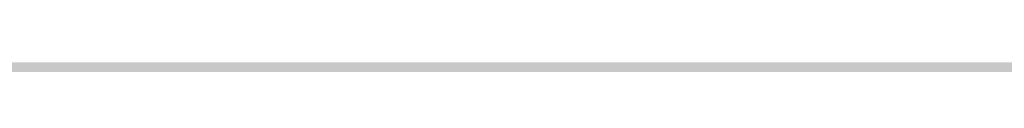
# Model space of a CAD drawing. Units: millimetres. Extents: x 0 to 2267, y 0 to 1823.
# Tile 207 of 256: x 1841.442 to 1842.748, y 1127.414 to 1127.416. Entities that reach past the tile are written whole.
import ezdxf

# ---------------------------------------------------------------- set-up
doc = ezdxf.new("R2010")
doc.units = ezdxf.units.MM
doc.header["$MEASUREMENT"] = 0
doc.layers.add('M-DIMS', color=2, linetype='Continuous', lineweight=25)
doc.layers.add('M-HATC', color=252, linetype='Continuous', lineweight=18)
doc.styles.get("Standard").update_dxf_attribs({"font": 'arial.ttf'})
doc.dimstyles.get("Standard").update_dxf_attribs({"dimtxt": 7, "dimasz": 4, "dimexe": 0.18, "dimexo": 0.0625, "dimgap": 0.09, "dimtad": 0, "dimdec": 0, "dimzin": 0, "dimdsep": 46, "dimtxsty": 'Standard', "dimcen": 0.09, "dimadec": 0, "dimazin": 0, "dimtfac": 1, "dimtdec": 0, "dimtofl": 0, "dimtmove": 0, "dimatfit": 3, "dimfxl": 1, "dimtolj": 1, "dimtzin": 0, "dimarcsym": 0})

# ---------------------------------------------------------------- blocks, each defined once
blk = doc.blocks.new('*D1')
at = {"layer": 'Defpoints', "color": 0, "transparency": 16777216}
for p in [(1593.4289, 1127.4171), (1843.4289, 1127.4171), (1843.4289, 955.6278)]:
    blk.add_point(p, dxfattribs=at)
at = {"layer": 'M-DIMS', "color": 0, "lineweight": -2, "transparency": 16777216}
for p, q in [((1593.4289, 1127.3546), (1593.4289, 955.4478)), ((1843.4289, 1127.3546), (1843.4289, 955.4478)), ((1597.4289, 955.6278), (1710.5582, 955.6278)), ((1839.4289, 955.6278), (1726.2996, 955.6278))]:
    blk.add_line(p, q, dxfattribs=at)
at = {"layer": 'M-DIMS', "color": 0, "transparency": 16777216}
for points in [[(1597.4289, 956.2944), (1597.4289, 954.9611), (1593.4289, 955.6278)], [(1839.4289, 956.2944), (1839.4289, 954.9611), (1843.4289, 955.6278)]]:
    blk.add_solid(points, dxfattribs=at)
at = {"layer": 'M-DIMS', "color": 0, "transparency": 16777216, "insert": (1718.4289, 955.6278), "char_height": 7, "attachment_point": 5}
blk.add_mtext('\\A1;250', dxfattribs=at)

msp = doc.modelspace()

# ---------------------------------------------------------------- hatches: boundary and pattern name
at = {"layer": 'M-HATC'}
h = msp.add_hatch(color=256, dxfattribs=at)
h.dxf.hatch_style = 1
h.paths.add_polyline_path([(2055.771, 1603.062), (1381.0868, 1603.062), (1381.0868, 1598.062), (2055.771, 1598.062)])
h.paths.add_polyline_path([(2055.771, 1598.062), (1381.0868, 1598.062), (1381.0868, 1593.062), (2055.771, 1593.062)])
h.paths.add_polyline_path([(2051.3074, 1536.7609), (1385.5504, 1536.7609), (1385.5504, 1526.7609), (1387.5504, 1526.7609), (1388.5366, 1525.0528), (1385.3319, 1521.2335), (1385.3319, 1521.2226), (2050.2542, 1522.7491), (2048.3212, 1525.0528), (2049.3074, 1526.7609), (2051.3074, 1526.7609)])
edge = h.paths.add_edge_path()
edge.add_arc((1847.5345, 1379.1492), 135, 222.603061, 222.890851, ccw=False)
edge.add_line((1748.1663, 1287.7656), (1683.0921, 1287.7656))
edge.add_arc((1583.7239, 1379.1492), 135, 317.109149, 317.396939, ccw=False)
edge.add_arc((1678.9686, 1290.6707), 5, 222.8909, 317.1091, ccw=False)
edge.add_arc((1774.2133, 1379.1492), 135, 222.603061, 222.890851, ccw=False)
edge.add_line((1674.8451, 1287.7656), (1609.7709, 1287.7656))
edge.add_arc((1510.4027, 1379.1492), 135, 317.109149, 317.396939, ccw=False)
edge.add_arc((1605.6474, 1290.6707), 5, 222.8909, 317.1091, ccw=False)
edge.add_arc((1700.8921, 1379.1492), 135, 222.603061, 222.890851, ccw=False)
edge.add_line((1601.5239, 1287.7656), (1536.4497, 1287.7656))
edge.add_arc((1437.0815, 1379.1492), 135, 317.109149, 317.396939, ccw=False)
edge.add_arc((1532.3262, 1290.6707), 5, 222.8909, 317.1091, ccw=False)
edge.add_arc((1627.5709, 1379.1492), 135, 222.603061, 222.890851, ccw=False)
edge.add_line((1528.2027, 1287.7656), (1505.9289, 1287.7656))
edge.add_spline(control_points=[(1505.9289, 1287.7656), (1504.2622, 1287.7656), (1504.2622, 1282.7656), (1505.9289, 1282.7656)], knot_values=[0, 0, 0, 0, 5, 5, 5, 5], degree=3, periodic=0)
edge.add_line((1505.9289, 1282.7656), (1930.9289, 1282.7656))
edge.add_spline(control_points=[(1930.9289, 1282.7656), (1932.5956, 1282.7656), (1932.5956, 1287.7656), (1930.9289, 1287.7656)], knot_values=[0, 0, 0, 0, 5, 5, 5, 5], degree=3, periodic=0)
edge.add_line((1930.9289, 1287.7656), (1903.0557, 1287.7656))
edge.add_arc((1803.6875, 1379.1492), 135, 317.109149, 317.396939, ccw=False)
edge.add_arc((1898.9322, 1290.6707), 5, 222.8909, 317.1091, ccw=False)
edge.add_arc((1994.1769, 1379.1492), 135, 222.603061, 222.890851, ccw=False)
edge.add_line((1894.8087, 1287.7656), (1829.7345, 1287.7656))
edge.add_arc((1730.3663, 1379.1492), 135, 317.109149, 317.396939, ccw=False)
edge.add_arc((1825.611, 1290.6707), 5, 222.8909, 317.1091, ccw=False)
edge.add_arc((1920.8557, 1379.1492), 135, 222.603061, 222.890851, ccw=False)
edge.add_line((1821.4875, 1287.7656), (1756.4133, 1287.7656))
edge.add_arc((1657.0451, 1379.1492), 135, 317.109149, 317.396939, ccw=False)
edge.add_arc((1752.2898, 1290.6707), 5, 222.8909, 317.1091, ccw=False)
edge = h.paths.add_edge_path()
edge.add_spline(control_points=[(1843.4289, 1227.2475), (1845.0956, 1227.2475), (1845.0956, 1232.2475), (1843.4289, 1232.2475)], knot_values=[0, 0, 0, 0, 5, 5, 5, 5], degree=3, periodic=0)
edge.add_line((1843.4289, 1232.2475), (1593.4289, 1232.2475))
edge.add_spline(control_points=[(1593.4289, 1232.2475), (1591.7622, 1232.2475), (1591.7622, 1227.2475), (1593.4289, 1227.2475)], knot_values=[0, 0, 0, 0, 5, 5, 5, 5], degree=3, periodic=0)
edge.add_line((1593.4289, 1227.2475), (1843.4289, 1227.2475))
h.paths.add_polyline_path([(1905.9289, 1127.4171), (1530.9289, 1127.4171, 0.414214), (1520.9289, 1117.4171), (1530.9289, 1117.4171), (1915.9289, 1117.4171, 0.414214)])
edge = h.paths.add_edge_path()
edge.add_arc((1397.0858, 1498.4078), 12.7299, 90.78215, 190.87871, ccw=False)
edge.add_line((1396.912, 1511.1365), (1428.0097, 1511.3488))
edge.add_line((1428.0097, 1511.3488), (1433.0097, 1511.3488))
edge.add_line((1433.0097, 1511.3488), (1434.439, 1511.3488))
edge.add_arc((1419.474, 1498.0804), 20, 41.561, 74.08211)
edge.add_line((1424.9592, 1517.3135), (1399.9351, 1517.2561))
edge.add_spline(control_points=[(1399.9307, 1517.2561), (1399.884, 1517.2131), (1399.8328, 1517.1689), (1399.7774, 1517.1236)], knot_values=[11.567499, 11.567499, 11.567499, 11.567499, 11.814249, 11.814249, 11.814249, 11.814249], degree=3, periodic=0)
edge.add_spline(control_points=[(1399.6328, 1517.0099), (1399.5831, 1516.9721), (1399.5307, 1516.9338), (1399.4759, 1516.8947)], knot_values=[11.167718, 11.167718, 11.167718, 11.167718, 11.365188, 11.365188, 11.365188, 11.365188], degree=3, periodic=0)
edge.add_spline(control_points=[(1399.3398, 1516.8001), (1399.1514, 1516.6719), (1398.9384, 1516.5377), (1398.704, 1516.3994)], knot_values=[10.376405, 10.376405, 10.376405, 10.376405, 11.00994, 11.00994, 11.00994, 11.00994], degree=3, periodic=0)
edge.add_spline(control_points=[(1398.6572, 1516.3719), (1398.5789, 1516.326), (1398.4983, 1516.2797), (1398.4155, 1516.2331)], knot_values=[10.125175, 10.125175, 10.125175, 10.125175, 10.334406, 10.334406, 10.334406, 10.334406], degree=3, periodic=0)
edge.add_spline(control_points=[(1398.2642, 1516.1487), (1398.196, 1516.1111), (1398.1263, 1516.0732), (1398.0555, 1516.0351)], knot_values=[9.832246, 9.832246, 9.832246, 9.832246, 9.999658, 9.999658, 9.999658, 9.999658], degree=3, periodic=0)
edge.add_spline(control_points=[(1397.9987, 1516.0048), (1397.7312, 1515.8621), (1397.446, 1515.7171), (1397.1466, 1515.5714)], knot_values=[9.161808, 9.161808, 9.161808, 9.161808, 9.787769, 9.787769, 9.787769, 9.787769], degree=3, periodic=0)
edge.add_spline(control_points=[(1397.1466, 1515.5714), (1396.8418, 1515.423), (1396.5222, 1515.274), (1396.1914, 1515.1262)], knot_values=[8.524455, 8.524455, 8.524455, 8.524455, 9.161808, 9.161808, 9.161808, 9.161808], degree=3, periodic=0)
edge.add_spline(control_points=[(1396.0777, 1515.0756), (1395.9854, 1515.0348), (1395.8922, 1514.994), (1395.7983, 1514.9534)], knot_values=[8.275193, 8.275193, 8.275193, 8.275193, 8.451726, 8.451726, 8.451726, 8.451726], degree=3, periodic=0)
edge.add_spline(control_points=[(1395.6018, 1514.8691), (1395.4997, 1514.8257), (1395.3968, 1514.7824), (1395.2932, 1514.7394)], knot_values=[7.962917, 7.962917, 7.962917, 7.962917, 8.152764, 8.152764, 8.152764, 8.152764], degree=3, periodic=0)
edge.add_spline(control_points=[(1395.2116, 1514.7057), (1394.8278, 1514.5475), (1394.4345, 1514.3929), (1394.0364, 1514.2442)], knot_values=[7.21254, 7.21254, 7.21254, 7.21254, 7.913148, 7.913148, 7.913148, 7.913148], degree=3, periodic=0)
edge.add_spline(control_points=[(1394.0364, 1514.2442), (1393.7076, 1514.1214), (1393.3754, 1514.0027), (1393.0427, 1513.8895)], knot_values=[6.633733, 6.633733, 6.633733, 6.633733, 7.21254, 7.21254, 7.21254, 7.21254], degree=3, periodic=0)
edge.add_spline(control_points=[(1392.8214, 1513.815), (1392.7198, 1513.7812), (1392.6181, 1513.7479), (1392.5166, 1513.7152)], knot_values=[6.328796, 6.328796, 6.328796, 6.328796, 6.505493, 6.505493, 6.505493, 6.505493], degree=3, periodic=0)
edge.add_spline(control_points=[(1392.5166, 1513.7152), (1392.3187, 1513.6515), (1392.1212, 1513.59), (1391.9244, 1513.531)], knot_values=[5.984605, 5.984605, 5.984605, 5.984605, 6.328796, 6.328796, 6.328796, 6.328796], degree=3, periodic=0)
edge.add_spline(control_points=[(1391.7915, 1513.4915), (1391.3122, 1513.3501), (1390.8384, 1513.2239), (1390.3784, 1513.1171)], knot_values=[5.066697, 5.066697, 5.066697, 5.066697, 5.907055, 5.907055, 5.907055, 5.907055], degree=3, periodic=0)
edge.add_spline(control_points=[(1390.3784, 1513.1171), (1390.1797, 1513.071), (1389.9836, 1513.0284), (1389.7907, 1512.9899)], knot_values=[4.70367, 4.70367, 4.70367, 4.70367, 5.066695, 5.066695, 5.066695, 5.066695], degree=3, periodic=0)
edge.add_spline(control_points=[(1389.422, 1512.9204), (1389.2459, 1512.8892), (1389.0729, 1512.8617), (1388.9036, 1512.8381)], knot_values=[4.130571, 4.130571, 4.130571, 4.130571, 4.469816, 4.469816, 4.469816, 4.469816], degree=3, periodic=0)
edge.add_spline(control_points=[(1388.9036, 1512.8381), (1388.591, 1512.7946), (1388.2911, 1512.7644), (1388.0071, 1512.7494)], knot_values=[3.504031, 3.504031, 3.504031, 3.504031, 4.130571, 4.130571, 4.130571, 4.130571], degree=3, periodic=0)
edge.add_spline(control_points=[(1387.9356, 1512.7459), (1387.8538, 1512.7423), (1387.7733, 1512.74), (1387.6944, 1512.739)], knot_values=[3.268866, 3.268866, 3.268866, 3.268866, 3.451164, 3.451164, 3.451164, 3.451164], degree=3, periodic=0)
edge.add_spline(control_points=[(1387.3351, 1512.7443), (1387.2076, 1512.7499), (1387.0847, 1512.7597), (1386.967, 1512.7739)], knot_values=[2.670686, 2.670686, 2.670686, 2.670686, 2.984, 2.984, 2.984, 2.984], degree=3, periodic=0)
edge.add_spline(control_points=[(1386.8327, 1512.7922), (1386.8209, 1512.7941), (1386.8092, 1512.7959), (1386.7975, 1512.7979)], knot_values=[2.516981, 2.516981, 2.516981, 2.516981, 2.549528, 2.549528, 2.549528, 2.549528], degree=3, periodic=0)
edge.add_spline(control_points=[(1386.4526, 1512.8735), (1386.4257, 1512.881), (1386.3993, 1512.889), (1386.3733, 1512.8972)], knot_values=[2.095869, 2.095869, 2.095869, 2.095869, 2.17941, 2.17941, 2.17941, 2.17941], degree=3, periodic=0)
edge.add_spline(control_points=[(1386.0691, 1513.0189), (1386.0634, 1513.0217), (1386.0577, 1513.0246), (1386.052, 1513.0275)], knot_values=[1.72453, 1.72453, 1.72453, 1.72453, 1.745933, 1.745933, 1.745933, 1.745933], degree=3, periodic=0)
edge.add_arc((1399.474, 1498.0804), 20, 131.82432, 180)
edge.add_arc((1630.3336, 1505.5484), 250.9708, 181.705176, 236.427975)
edge.add_arc((1605.3399, 1483.3044), 218.7822, 238.660829, 243.34961)
edge.add_arc((1647.0911, 1510.3592), 262.8986, 183.129836, 237.853442, ccw=False)
h.paths.add_polyline_path([(1406.5369, 1391.9644, 0.149382), (1491.5506, 1296.4418, -0.129517)], flags=17)
edge = h.paths.add_edge_path()
edge.add_arc((2037.3838, 1498.0804), 20, 0, 48.26587)
edge.add_spline(control_points=[(2050.6973, 1513.0052), (2050.6512, 1512.9847), (2050.6034, 1512.9655), (2050.5539, 1512.9477)], knot_values=[1.835652, 1.835652, 1.835652, 1.835652, 2.000781, 2.000781, 2.000781, 2.000781], degree=3, periodic=0)
edge.add_spline(control_points=[(2050.4616, 1512.9166), (2050.479, 1512.9221), (2050.4963, 1512.9277), (2050.5133, 1512.9335)], knot_values=[2.045477, 2.045477, 2.045477, 2.045477, 2.101389, 2.101389, 2.101389, 2.101389], degree=3, periodic=0)
edge.add_spline(control_points=[(2050.129, 1512.8342), (2050.1984, 1512.8473), (2050.2657, 1512.8623), (2050.3308, 1512.8792)], knot_values=[2.237629, 2.237629, 2.237629, 2.237629, 2.435841, 2.435841, 2.435841, 2.435841], degree=3, periodic=0)
edge.add_spline(control_points=[(2050.0946, 1512.8278), (2050.1061, 1512.8299), (2050.1176, 1512.832), (2050.129, 1512.8342)], knot_values=[2.435841, 2.435841, 2.435841, 2.435841, 2.468321, 2.468321, 2.468321, 2.468321], degree=3, periodic=0)
edge.add_spline(control_points=[(2049.7843, 1512.7851), (2049.8552, 1512.7922), (2049.9243, 1512.8008), (2049.9917, 1512.8109)], knot_values=[2.563852, 2.563852, 2.563852, 2.563852, 2.748541, 2.748541, 2.748541, 2.748541], degree=3, periodic=0)
edge.add_spline(control_points=[(2049.4052, 1512.7617), (2049.5364, 1512.7653), (2049.6629, 1512.773), (2049.7843, 1512.7851)], knot_values=[2.748541, 2.748541, 2.748541, 2.748541, 3.064882, 3.064882, 3.064882, 3.064882], degree=3, periodic=0)
edge.add_spline(control_points=[(2049.1698, 1512.7597), (2049.2336, 1512.7591), (2049.2965, 1512.7594), (2049.3584, 1512.7606)], knot_values=[3.102309, 3.102309, 3.102309, 3.102309, 3.2503, 3.2503, 3.2503, 3.2503], degree=3, periodic=0)
edge.add_spline(control_points=[(2048.8573, 1512.7691), (2048.9638, 1512.7638), (2049.068, 1512.7606), (2049.1698, 1512.7597)], knot_values=[3.2503, 3.2503, 3.2503, 3.2503, 3.486069, 3.486069, 3.486069, 3.486069], degree=3, periodic=0)
edge.add_spline(control_points=[(2048.6924, 1512.7789), (2048.3729, 1512.8009), (2048.0345, 1512.8411), (2047.6817, 1512.897)], knot_values=[3.606429, 3.606429, 3.606429, 3.606429, 4.2989, 4.2989, 4.2989, 4.2989], degree=3, periodic=0)
edge.add_spline(control_points=[(2047.6817, 1512.897), (2047.5458, 1512.9185), (2047.4077, 1512.9424), (2047.2678, 1512.9685)], knot_values=[4.2989, 4.2989, 4.2989, 4.2989, 4.565769, 4.565769, 4.565769, 4.565769], degree=3, periodic=0)
edge.add_spline(control_points=[(2047.2678, 1512.9685), (2047.1449, 1512.9914), (2047.0207, 1513.016), (2046.8951, 1513.0422)], knot_values=[4.565769, 4.565769, 4.565769, 4.565769, 4.799971, 4.799971, 4.799971, 4.799971], degree=3, periodic=0)
edge.add_spline(control_points=[(2046.8951, 1513.0422), (2046.5286, 1513.1188), (2046.1513, 1513.209), (2045.7676, 1513.3107)], knot_values=[4.799971, 4.799971, 4.799971, 4.799971, 5.483718, 5.483718, 5.483718, 5.483718], degree=3, periodic=0)
edge.add_spline(control_points=[(2045.7676, 1513.3107), (2045.3724, 1513.4154), (2044.9704, 1513.5322), (2044.5662, 1513.6588)], knot_values=[5.483718, 5.483718, 5.483718, 5.483718, 6.187866, 6.187866, 6.187866, 6.187866], degree=3, periodic=0)
edge.add_spline(control_points=[(2044.5662, 1513.6588), (2044.4149, 1513.7061), (2044.2633, 1513.7549), (2044.1116, 1513.8048)], knot_values=[6.187866, 6.187866, 6.187866, 6.187866, 6.451551, 6.451551, 6.451551, 6.451551], degree=3, periodic=0)
edge.add_spline(control_points=[(2044.1116, 1513.8048), (2043.9967, 1513.8427), (2043.8817, 1513.8813), (2043.7668, 1513.9205)], knot_values=[6.451551, 6.451551, 6.451551, 6.451551, 6.651434, 6.651434, 6.651434, 6.651434], degree=3, periodic=0)
edge.add_spline(control_points=[(2043.7668, 1513.9205), (2043.3716, 1514.0554), (2042.9774, 1514.1979), (2042.5886, 1514.3458)], knot_values=[6.651434, 6.651434, 6.651434, 6.651434, 7.338879, 7.338879, 7.338879, 7.338879], degree=3, periodic=0)
edge.add_spline(control_points=[(2042.5886, 1514.3458), (2042.1643, 1514.5071), (2041.7465, 1514.6749), (2041.3409, 1514.846)], knot_values=[7.338879, 7.338879, 7.338879, 7.338879, 8.089209, 8.089209, 8.089209, 8.089209], degree=3, periodic=0)
edge.add_spline(control_points=[(2041.3409, 1514.846), (2041.1028, 1514.9465), (2040.869, 1515.0481), (2040.6405, 1515.1502)], knot_values=[8.089209, 8.089209, 8.089209, 8.089209, 8.529587, 8.529587, 8.529587, 8.529587], degree=3, periodic=0)
edge.add_spline(control_points=[(2040.51, 1515.2089), (2040.0824, 1515.4022), (2039.6747, 1515.5971), (2039.295, 1515.7894)], knot_values=[8.613818, 8.613818, 8.613818, 8.613818, 9.44571, 9.44571, 9.44571, 9.44571], degree=3, periodic=0)
edge.add_spline(control_points=[(2039.295, 1515.7894), (2039.0618, 1515.9075), (2038.8391, 1516.0246), (2038.6288, 1516.1398)], knot_values=[9.44571, 9.44571, 9.44571, 9.44571, 9.956404, 9.956404, 9.956404, 9.956404], degree=3, periodic=0)
edge.add_spline(control_points=[(2038.6288, 1516.1398), (2038.5187, 1516.2001), (2038.4121, 1516.2598), (2038.309, 1516.3189)], knot_values=[9.956404, 9.956404, 9.956404, 9.956404, 10.223542, 10.223542, 10.223542, 10.223542], degree=3, periodic=0)
edge.add_spline(control_points=[(2038.309, 1516.3189), (2038.2138, 1516.3735), (2038.1216, 1516.4276), (2038.0328, 1516.481)], knot_values=[10.223542, 10.223542, 10.223542, 10.223542, 10.47051, 10.47051, 10.47051, 10.47051], degree=3, periodic=0)
edge.add_spline(control_points=[(2038.0328, 1516.481), (2037.7855, 1516.6296), (2037.5639, 1516.773), (2037.3722, 1516.909)], knot_values=[10.47051, 10.47051, 10.47051, 10.47051, 11.15767, 11.15767, 11.15767, 11.15767], degree=3, periodic=0)
edge.add_spline(control_points=[(2037.3722, 1516.909), (2037.2789, 1516.9752), (2037.1927, 1517.0396), (2037.1142, 1517.102)], knot_values=[11.15767, 11.15767, 11.15767, 11.15767, 11.49227, 11.49227, 11.49227, 11.49227], degree=3, periodic=0)
edge.add_spline(control_points=[(2036.8564, 1517.3259), (2036.9148, 1517.2692), (2036.9814, 1517.2103), (2037.0557, 1517.1492)], knot_values=[11.577341, 11.577341, 11.577341, 11.577341, 11.91035, 11.91035, 11.91035, 11.91035], degree=3, periodic=0)
edge.add_spline(control_points=[(2036.8074, 1517.3748), (2036.823, 1517.3587), (2036.8393, 1517.3424), (2036.8564, 1517.3259)], knot_values=[11.91035, 11.91035, 11.91035, 11.91035, 12.007402, 12.007402, 12.007402, 12.007402], degree=3, periodic=0)
edge.add_spline(control_points=[(2036.7017, 1517.494), (2036.7104, 1517.483), (2036.7196, 1517.4719), (2036.7291, 1517.4606)], knot_values=[12.184155, 12.184155, 12.184155, 12.184155, 12.255409, 12.255409, 12.255409, 12.255409], degree=3, periodic=0)
edge.add_spline(control_points=[(2036.6159, 1517.6205), (2036.62, 1517.613), (2036.6243, 1517.6055), (2036.6289, 1517.5979)], knot_values=[12.487913, 12.487913, 12.487913, 12.487913, 12.541035, 12.541035, 12.541035, 12.541035], degree=3, periodic=0)
edge.add_spline(control_points=[(2036.5635, 1517.786), (2036.5637, 1517.7794), (2036.5642, 1517.7726), (2036.565, 1517.7658)], knot_values=[12.911761, 12.911761, 12.911761, 12.911761, 12.968286, 12.968286, 12.968286, 12.968286], degree=3, periodic=0)
edge.add_spline(control_points=[(2036.6166, 1517.9304), (2036.6125, 1517.9259), (2036.6086, 1517.9212), (2036.6049, 1517.9165)], knot_values=[13.382527, 13.382527, 13.382527, 13.382527, 13.433791, 13.433791, 13.433791, 13.433791], degree=3, periodic=0)
edge.add_spline(control_points=[(2036.749, 1518.017), (2036.7361, 1518.0116), (2036.7239, 1518.006), (2036.7124, 1518.0002)], knot_values=[13.726299, 13.726299, 13.726299, 13.726299, 13.809928, 13.809928, 13.809928, 13.809928], degree=3, periodic=0)
edge.add_spline(control_points=[(2036.8604, 1518.0528), (2036.8386, 1518.0474), (2036.8181, 1518.0416), (2036.7988, 1518.0353)], knot_values=[13.910887, 13.910887, 13.910887, 13.910887, 14.02153, 14.02153, 14.02153, 14.02153], degree=3, periodic=0)
edge.add_line((2036.9639, 1518.0804), (2032.3838, 1518.0804))
edge.add_line((2032.3838, 1518.0804), (2027.3838, 1518.0804))
edge.add_line((2027.3838, 1518.0804), (2022.3838, 1518.0804))
edge.add_line((2022.3838, 1518.0804), (2017.3838, 1518.0804))
edge.add_arc((2017.3838, 1498.0804), 20, 90, 138.439)
edge.add_line((2002.4188, 1511.3488), (2003.8481, 1511.3488))
edge.add_line((2003.8481, 1511.3488), (2008.8481, 1511.3488))
edge.add_line((2008.8481, 1511.3488), (2039.772, 1511.1377))
edge.add_arc((2039.772, 1498.4078), 12.7299, -10.87871, 90, ccw=False)
edge.add_arc((1789.7668, 1510.3592), 262.8986, 302.146558, 356.870164, ccw=False)
edge.add_arc((1831.5179, 1483.3044), 218.7822, 296.65039, 301.339171)
edge.add_arc((1806.5242, 1505.5484), 250.9708, 303.572025, 358.294824)
h.paths.add_polyline_path([(2030.321, 1391.9644, -0.129517), (1945.3072, 1296.4418, 0.149382)], flags=17)
edge = h.paths.add_edge_path()
edge.add_spline(control_points=[(2037.2464, 1518.0821), (2037.2898, 1518.081), (2037.3355, 1518.0804), (2037.3838, 1518.0804)], knot_values=[0.000012, 0.000012, 0.000012, 0.000012, 0.144754, 0.144754, 0.144754, 0.144754], degree=3, periodic=0)
edge.add_line((2037.3357, 1518.0804), (2037.0096, 1518.0804))
edge.add_spline(control_points=[(2037.0096, 1518.0804), (2036.9822, 1518.0768), (2036.956, 1518.0727), (2036.9312, 1518.0681)], knot_values=[14.13465, 14.13465, 14.13465, 14.13465, 14.247197, 14.247197, 14.247197, 14.247197], degree=3, periodic=0)
edge.add_spline(control_points=[(2036.9312, 1518.0681), (2036.9276, 1518.0674), (2036.9241, 1518.0667), (2036.9205, 1518.0661)], knot_values=[14.118315, 14.118315, 14.118315, 14.118315, 14.13465, 14.13465, 14.13465, 14.13465], degree=3, periodic=0)
edge.add_spline(control_points=[(2036.9205, 1518.0661), (2036.9118, 1518.0644), (2036.9032, 1518.0626), (2036.8948, 1518.0608)], knot_values=[14.078086, 14.078086, 14.078086, 14.078086, 14.118315, 14.118315, 14.118315, 14.118315], degree=3, periodic=0)
edge.add_spline(control_points=[(2036.8948, 1518.0608), (2036.883, 1518.0583), (2036.8716, 1518.0556), (2036.8604, 1518.0528)], knot_values=[14.02153, 14.02153, 14.02153, 14.02153, 14.078086, 14.078086, 14.078086, 14.078086], degree=3, periodic=0)
edge.add_spline(control_points=[(2036.8604, 1518.0528), (2036.8386, 1518.0474), (2036.8181, 1518.0416), (2036.7988, 1518.0353)], knot_values=[13.910887, 13.910887, 13.910887, 13.910887, 14.02153, 14.02153, 14.02153, 14.02153], degree=3, periodic=0)
edge.add_spline(control_points=[(2036.7988, 1518.0353), (2036.7981, 1518.035), (2036.7974, 1518.0348), (2036.7967, 1518.0346)], knot_values=[13.906906, 13.906906, 13.906906, 13.906906, 13.910887, 13.910887, 13.910887, 13.910887], degree=3, periodic=0)
edge.add_spline(control_points=[(2036.7967, 1518.0346), (2036.7882, 1518.0318), (2036.7799, 1518.0289), (2036.7719, 1518.0259)], knot_values=[13.857826, 13.857826, 13.857826, 13.857826, 13.906906, 13.906906, 13.906906, 13.906906], degree=3, periodic=0)
edge.add_spline(control_points=[(2036.7719, 1518.0259), (2036.764, 1518.023), (2036.7564, 1518.02), (2036.749, 1518.017)], knot_values=[13.809928, 13.809928, 13.809928, 13.809928, 13.857826, 13.857826, 13.857826, 13.857826], degree=3, periodic=0)
edge.add_spline(control_points=[(2036.749, 1518.017), (2036.7361, 1518.0116), (2036.7239, 1518.006), (2036.7124, 1518.0002)], knot_values=[13.726299, 13.726299, 13.726299, 13.726299, 13.809928, 13.809928, 13.809928, 13.809928], degree=3, periodic=0)
edge.add_spline(control_points=[(2036.7124, 1518.0002), (2036.7121, 1518), (2036.7118, 1517.9999), (2036.7115, 1517.9997)], knot_values=[13.723993, 13.723993, 13.723993, 13.723993, 13.726299, 13.726299, 13.726299, 13.726299], degree=3, periodic=0)
edge.add_spline(control_points=[(2036.7115, 1517.9997), (2036.7063, 1517.9971), (2036.7013, 1517.9944), (2036.6965, 1517.9917)], knot_values=[13.686536, 13.686536, 13.686536, 13.686536, 13.723993, 13.723993, 13.723993, 13.723993], degree=3, periodic=0)
edge.add_spline(control_points=[(2036.6965, 1517.9917), (2036.6919, 1517.9891), (2036.6874, 1517.9865), (2036.6831, 1517.9839)], knot_values=[13.651251, 13.651251, 13.651251, 13.651251, 13.686536, 13.686536, 13.686536, 13.686536], degree=3, periodic=0)
edge.add_spline(control_points=[(2036.6831, 1517.9839), (2036.6764, 1517.9798), (2036.67, 1517.9757), (2036.6639, 1517.9714)], knot_values=[13.596804, 13.596804, 13.596804, 13.596804, 13.651251, 13.651251, 13.651251, 13.651251], degree=3, periodic=0)
edge.add_spline(control_points=[(2036.6639, 1517.9714), (2036.6636, 1517.9712), (2036.6633, 1517.9709), (2036.6629, 1517.9707)], knot_values=[13.593956, 13.593956, 13.593956, 13.593956, 13.596804, 13.596804, 13.596804, 13.596804], degree=3, periodic=0)
edge.add_spline(control_points=[(2036.6629, 1517.9707), (2036.6603, 1517.9689), (2036.6577, 1517.967), (2036.6552, 1517.9651)], knot_values=[13.570322, 13.570322, 13.570322, 13.570322, 13.593956, 13.593956, 13.593956, 13.593956], degree=3, periodic=0)
edge.add_spline(control_points=[(2036.6552, 1517.9651), (2036.6525, 1517.9631), (2036.6499, 1517.9611), (2036.6474, 1517.9591)], knot_values=[13.545477, 13.545477, 13.545477, 13.545477, 13.570322, 13.570322, 13.570322, 13.570322], degree=3, periodic=0)
edge.add_spline(control_points=[(2036.6474, 1517.9591), (2036.6472, 1517.9589), (2036.6471, 1517.9588), (2036.6469, 1517.9587)], knot_values=[13.543931, 13.543931, 13.543931, 13.543931, 13.545477, 13.545477, 13.545477, 13.545477], degree=3, periodic=0)
edge.add_spline(control_points=[(2036.6469, 1517.9587), (2036.6412, 1517.9541), (2036.6358, 1517.9494), (2036.6307, 1517.9447)], knot_values=[13.488237, 13.488237, 13.488237, 13.488237, 13.543931, 13.543931, 13.543931, 13.543931], degree=3, periodic=0)
edge.add_spline(control_points=[(2036.6307, 1517.9447), (2036.6282, 1517.9423), (2036.6257, 1517.9399), (2036.6233, 1517.9374)], knot_values=[13.460307, 13.460307, 13.460307, 13.460307, 13.488237, 13.488237, 13.488237, 13.488237], degree=3, periodic=0)
edge.add_spline(control_points=[(2036.6233, 1517.9374), (2036.6215, 1517.9356), (2036.6198, 1517.9338), (2036.6181, 1517.932)], knot_values=[13.439712, 13.439712, 13.439712, 13.439712, 13.460307, 13.460307, 13.460307, 13.460307], degree=3, periodic=0)
edge.add_spline(control_points=[(2036.6181, 1517.932), (2036.6176, 1517.9315), (2036.6171, 1517.9309), (2036.6166, 1517.9304)], knot_values=[13.433791, 13.433791, 13.433791, 13.433791, 13.439712, 13.439712, 13.439712, 13.439712], degree=3, periodic=0)
edge.add_spline(control_points=[(2036.6166, 1517.9304), (2036.6125, 1517.9259), (2036.6086, 1517.9212), (2036.6049, 1517.9165)], knot_values=[13.382527, 13.382527, 13.382527, 13.382527, 13.433791, 13.433791, 13.433791, 13.433791], degree=3, periodic=0)
edge.add_spline(control_points=[(2036.6049, 1517.9165), (2036.6026, 1517.9135), (2036.6004, 1517.9104), (2036.5982, 1517.9074)], knot_values=[13.350017, 13.350017, 13.350017, 13.350017, 13.382527, 13.382527, 13.382527, 13.382527], degree=3, periodic=0)
edge.add_spline(control_points=[(2036.5982, 1517.9074), (2036.5972, 1517.9059), (2036.5962, 1517.9043), (2036.5952, 1517.9028)], knot_values=[13.333922, 13.333922, 13.333922, 13.333922, 13.350017, 13.350017, 13.350017, 13.350017], degree=3, periodic=0)
edge.add_spline(control_points=[(2036.5952, 1517.9028), (2036.5945, 1517.9018), (2036.5939, 1517.9009), (2036.5933, 1517.8999)], knot_values=[13.323828, 13.323828, 13.323828, 13.323828, 13.333922, 13.333922, 13.333922, 13.333922], degree=3, periodic=0)
edge.add_spline(control_points=[(2036.5933, 1517.8999), (2036.5905, 1517.8955), (2036.5879, 1517.8909), (2036.5855, 1517.8864)], knot_values=[13.277545, 13.277545, 13.277545, 13.277545, 13.323828, 13.323828, 13.323828, 13.323828], degree=3, periodic=0)
edge.add_spline(control_points=[(2036.5855, 1517.8864), (2036.5836, 1517.8827), (2036.5817, 1517.8789), (2036.5801, 1517.8751)], knot_values=[13.240119, 13.240119, 13.240119, 13.240119, 13.277545, 13.277545, 13.277545, 13.277545], degree=3, periodic=0)
edge.add_spline(control_points=[(2036.5801, 1517.8751), (2036.5795, 1517.8739), (2036.579, 1517.8727), (2036.5785, 1517.8715)], knot_values=[13.228211, 13.228211, 13.228211, 13.228211, 13.240119, 13.240119, 13.240119, 13.240119], degree=3, periodic=0)
edge.add_spline(control_points=[(2036.5785, 1517.8715), (2036.578, 1517.8702), (2036.5774, 1517.869), (2036.5769, 1517.8677)], knot_values=[13.215717, 13.215717, 13.215717, 13.215717, 13.228211, 13.228211, 13.228211, 13.228211], degree=3, periodic=0)
edge.add_spline(control_points=[(2036.5769, 1517.8677), (2036.5755, 1517.864), (2036.5741, 1517.8603), (2036.5729, 1517.8565)], knot_values=[13.179847, 13.179847, 13.179847, 13.179847, 13.215717, 13.215717, 13.215717, 13.215717], degree=3, periodic=0)
edge.add_spline(control_points=[(2036.5729, 1517.8565), (2036.5713, 1517.8515), (2036.5699, 1517.8464), (2036.5687, 1517.8413)], knot_values=[13.132017, 13.132017, 13.132017, 13.132017, 13.179847, 13.179847, 13.179847, 13.179847], degree=3, periodic=0)
edge.add_spline(control_points=[(2036.5687, 1517.8413), (2036.5684, 1517.8402), (2036.5682, 1517.8392), (2036.568, 1517.8382)], knot_values=[13.122482, 13.122482, 13.122482, 13.122482, 13.132017, 13.132017, 13.132017, 13.132017], degree=3, periodic=0)
edge.add_spline(control_points=[(2036.568, 1517.8382), (2036.5676, 1517.8363), (2036.5672, 1517.8345), (2036.5669, 1517.8327)], knot_values=[13.105592, 13.105592, 13.105592, 13.105592, 13.122482, 13.122482, 13.122482, 13.122482], degree=3, periodic=0)
edge.add_spline(control_points=[(2036.5669, 1517.8327), (2036.5662, 1517.8292), (2036.5657, 1517.8257), (2036.5652, 1517.8222)], knot_values=[13.074063, 13.074063, 13.074063, 13.074063, 13.105592, 13.105592, 13.105592, 13.105592], degree=3, periodic=0)
edge.add_spline(control_points=[(2036.5652, 1517.8222), (2036.5652, 1517.8222), (2036.5652, 1517.8222), (2036.5652, 1517.8222)], knot_values=[13.074043, 13.074043, 13.074043, 13.074043, 13.074063, 13.074063, 13.074063, 13.074063], degree=3, periodic=0)
edge.add_spline(control_points=[(2036.5652, 1517.8222), (2036.5644, 1517.8164), (2036.5639, 1517.8106), (2036.5636, 1517.8046)], knot_values=[13.021884, 13.021884, 13.021884, 13.021884, 13.074043, 13.074043, 13.074043, 13.074043], degree=3, periodic=0)
edge.add_spline(control_points=[(2036.5636, 1517.8046), (2036.5636, 1517.804), (2036.5636, 1517.8034), (2036.5635, 1517.8028)], knot_values=[13.01674, 13.01674, 13.01674, 13.01674, 13.021884, 13.021884, 13.021884, 13.021884], degree=3, periodic=0)
edge.add_spline(control_points=[(2036.5635, 1517.8028), (2036.5634, 1517.8005), (2036.5634, 1517.7982), (2036.5634, 1517.7958)], knot_values=[12.996438, 12.996438, 12.996438, 12.996438, 13.01674, 13.01674, 13.01674, 13.01674], degree=3, periodic=0)
edge.add_spline(control_points=[(2036.5634, 1517.7958), (2036.5633, 1517.7926), (2036.5634, 1517.7893), (2036.5635, 1517.786)], knot_values=[12.968286, 12.968286, 12.968286, 12.968286, 12.996438, 12.996438, 12.996438, 12.996438], degree=3, periodic=0)
edge.add_spline(control_points=[(2036.5635, 1517.786), (2036.5637, 1517.7794), (2036.5642, 1517.7726), (2036.565, 1517.7658)], knot_values=[12.911761, 12.911761, 12.911761, 12.911761, 12.968286, 12.968286, 12.968286, 12.968286], degree=3, periodic=0)
edge.add_spline(control_points=[(2036.565, 1517.7658), (2036.565, 1517.7657), (2036.565, 1517.7656), (2036.565, 1517.7656)], knot_values=[12.911017, 12.911017, 12.911017, 12.911017, 12.911761, 12.911761, 12.911761, 12.911761], degree=3, periodic=0)
edge.add_spline(control_points=[(2036.565, 1517.7656), (2036.5654, 1517.7625), (2036.5658, 1517.7593), (2036.5663, 1517.7562)], knot_values=[12.88528, 12.88528, 12.88528, 12.88528, 12.911017, 12.911017, 12.911017, 12.911017], degree=3, periodic=0)
edge.add_spline(control_points=[(2036.5663, 1517.7562), (2036.5667, 1517.7534), (2036.5672, 1517.7506), (2036.5677, 1517.7478)], knot_values=[12.862519, 12.862519, 12.862519, 12.862519, 12.88528, 12.88528, 12.88528, 12.88528], degree=3, periodic=0)
edge.add_spline(control_points=[(2036.5677, 1517.7478), (2036.5678, 1517.7474), (2036.5679, 1517.7469), (2036.568, 1517.7465)], knot_values=[12.858885, 12.858885, 12.858885, 12.858885, 12.862519, 12.862519, 12.862519, 12.862519], degree=3, periodic=0)
edge.add_spline(control_points=[(2036.568, 1517.7465), (2036.5692, 1517.7399), (2036.5707, 1517.7332), (2036.5724, 1517.7264)], knot_values=[12.8053, 12.8053, 12.8053, 12.8053, 12.858885, 12.858885, 12.858885, 12.858885], degree=3, periodic=0)
edge.add_spline(control_points=[(2036.5724, 1517.7264), (2036.5734, 1517.7226), (2036.5745, 1517.7187), (2036.5756, 1517.7149)], knot_values=[12.775176, 12.775176, 12.775176, 12.775176, 12.8053, 12.8053, 12.8053, 12.8053], degree=3, periodic=0)
edge.add_spline(control_points=[(2036.5756, 1517.7149), (2036.5763, 1517.7125), (2036.577, 1517.7102), (2036.5778, 1517.7078)], knot_values=[12.756759, 12.756759, 12.756759, 12.756759, 12.775176, 12.775176, 12.775176, 12.775176], degree=3, periodic=0)
edge.add_spline(control_points=[(2036.5778, 1517.7078), (2036.5781, 1517.7067), (2036.5784, 1517.7057), (2036.5787, 1517.7047)], knot_values=[12.748742, 12.748742, 12.748742, 12.748742, 12.756759, 12.756759, 12.756759, 12.756759], degree=3, periodic=0)
edge.add_spline(control_points=[(2036.5787, 1517.7047), (2036.5808, 1517.6983), (2036.5831, 1517.6919), (2036.5856, 1517.6854)], knot_values=[12.69959, 12.69959, 12.69959, 12.69959, 12.748742, 12.748742, 12.748742, 12.748742], degree=3, periodic=0)
edge.add_spline(control_points=[(2036.5856, 1517.6854), (2036.5876, 1517.68), (2036.5898, 1517.6746), (2036.5921, 1517.6692)], knot_values=[12.659038, 12.659038, 12.659038, 12.659038, 12.69959, 12.69959, 12.69959, 12.69959], degree=3, periodic=0)
edge.add_spline(control_points=[(2036.5921, 1517.6692), (2036.594, 1517.6648), (2036.5959, 1517.6605), (2036.5979, 1517.6561)], knot_values=[12.626806, 12.626806, 12.626806, 12.626806, 12.659038, 12.659038, 12.659038, 12.659038], degree=3, periodic=0)
edge.add_spline(control_points=[(2036.5979, 1517.6561), (2036.5984, 1517.6551), (2036.5989, 1517.6541), (2036.5993, 1517.6531)], knot_values=[12.619394, 12.619394, 12.619394, 12.619394, 12.626806, 12.626806, 12.626806, 12.626806], degree=3, periodic=0)
edge.add_spline(control_points=[(2036.5993, 1517.6531), (2036.6043, 1517.6424), (2036.6099, 1517.6315), (2036.6159, 1517.6205)], knot_values=[12.541039, 12.541039, 12.541039, 12.541039, 12.619394, 12.619394, 12.619394, 12.619394], degree=3, periodic=0)
edge.add_spline(control_points=[(2036.6159, 1517.6205), (2036.6159, 1517.6205), (2036.6159, 1517.6205), (2036.6159, 1517.6205)], knot_values=[12.541035, 12.541035, 12.541035, 12.541035, 12.541039, 12.541039, 12.541039, 12.541039], degree=3, periodic=0)
edge.add_spline(control_points=[(2036.6159, 1517.6205), (2036.62, 1517.613), (2036.6243, 1517.6055), (2036.6289, 1517.5979)], knot_values=[12.487913, 12.487913, 12.487913, 12.487913, 12.541035, 12.541035, 12.541035, 12.541035], degree=3, periodic=0)
edge.add_spline(control_points=[(2036.6289, 1517.5979), (2036.6326, 1517.5916), (2036.6365, 1517.5853), (2036.6406, 1517.5789)], knot_values=[12.443982, 12.443982, 12.443982, 12.443982, 12.487913, 12.487913, 12.487913, 12.487913], degree=3, periodic=0)
edge.add_spline(control_points=[(2036.6406, 1517.5789), (2036.6414, 1517.5776), (2036.6423, 1517.5763), (2036.6431, 1517.5749)], knot_values=[12.434996, 12.434996, 12.434996, 12.434996, 12.443982, 12.443982, 12.443982, 12.443982], degree=3, periodic=0)
edge.add_spline(control_points=[(2036.6431, 1517.5749), (2036.6531, 1517.5596), (2036.6639, 1517.5439), (2036.6756, 1517.528)], knot_values=[12.329647, 12.329647, 12.329647, 12.329647, 12.434996, 12.434996, 12.434996, 12.434996], degree=3, periodic=0)
edge.add_spline(control_points=[(2036.6756, 1517.528), (2036.6839, 1517.5168), (2036.6925, 1517.5055), (2036.7017, 1517.494)], knot_values=[12.255409, 12.255409, 12.255409, 12.255409, 12.329647, 12.329647, 12.329647, 12.329647], degree=3, periodic=0)
edge.add_spline(control_points=[(2036.7017, 1517.494), (2036.7104, 1517.483), (2036.7196, 1517.4719), (2036.7291, 1517.4606)], knot_values=[12.184155, 12.184155, 12.184155, 12.184155, 12.255409, 12.255409, 12.255409, 12.255409], degree=3, periodic=0)
edge.add_spline(control_points=[(2036.7291, 1517.4606), (2036.7436, 1517.4435), (2036.759, 1517.4262), (2036.7753, 1517.4085)], knot_values=[12.075961, 12.075961, 12.075961, 12.075961, 12.184155, 12.184155, 12.184155, 12.184155], degree=3, periodic=0)
edge.add_spline(control_points=[(2036.7753, 1517.4085), (2036.7763, 1517.4075), (2036.7773, 1517.4064), (2036.7783, 1517.4054)], knot_values=[12.069502, 12.069502, 12.069502, 12.069502, 12.075961, 12.075961, 12.075961, 12.075961], degree=3, periodic=0)
edge.add_spline(control_points=[(2036.7783, 1517.4054), (2036.7877, 1517.3953), (2036.7974, 1517.385), (2036.8074, 1517.3748)], knot_values=[12.007402, 12.007402, 12.007402, 12.007402, 12.069502, 12.069502, 12.069502, 12.069502], degree=3, periodic=0)
edge.add_spline(control_points=[(2036.8074, 1517.3748), (2036.823, 1517.3587), (2036.8393, 1517.3424), (2036.8564, 1517.3259)], knot_values=[11.91035, 11.91035, 11.91035, 11.91035, 12.007402, 12.007402, 12.007402, 12.007402], degree=3, periodic=0)
edge.add_spline(control_points=[(2036.8564, 1517.3259), (2036.9148, 1517.2692), (2036.9814, 1517.2103), (2037.0557, 1517.1492)], knot_values=[11.577341, 11.577341, 11.577341, 11.577341, 11.91035, 11.91035, 11.91035, 11.91035], degree=3, periodic=0)
edge.add_spline(control_points=[(2037.0557, 1517.1492), (2037.0747, 1517.1336), (2037.0942, 1517.1179), (2037.1142, 1517.102)], knot_values=[11.49227, 11.49227, 11.49227, 11.49227, 11.577341, 11.577341, 11.577341, 11.577341], degree=3, periodic=0)
edge.add_spline(control_points=[(2037.1142, 1517.102), (2037.1927, 1517.0396), (2037.2789, 1516.9752), (2037.3722, 1516.909)], knot_values=[11.15767, 11.15767, 11.15767, 11.15767, 11.49227, 11.49227, 11.49227, 11.49227], degree=3, periodic=0)
edge.add_spline(control_points=[(2037.3722, 1516.909), (2037.5639, 1516.773), (2037.7855, 1516.6296), (2038.0328, 1516.481)], knot_values=[10.47051, 10.47051, 10.47051, 10.47051, 11.15767, 11.15767, 11.15767, 11.15767], degree=3, periodic=0)
edge.add_spline(control_points=[(2038.0328, 1516.481), (2038.1216, 1516.4276), (2038.2138, 1516.3735), (2038.309, 1516.3189)], knot_values=[10.223542, 10.223542, 10.223542, 10.223542, 10.47051, 10.47051, 10.47051, 10.47051], degree=3, periodic=0)
edge.add_spline(control_points=[(2038.309, 1516.3189), (2038.4121, 1516.2598), (2038.5187, 1516.2001), (2038.6288, 1516.1398)], knot_values=[9.956404, 9.956404, 9.956404, 9.956404, 10.223542, 10.223542, 10.223542, 10.223542], degree=3, periodic=0)
edge.add_spline(control_points=[(2038.6288, 1516.1398), (2038.8391, 1516.0246), (2039.0618, 1515.9075), (2039.295, 1515.7894)], knot_values=[9.44571, 9.44571, 9.44571, 9.44571, 9.956404, 9.956404, 9.956404, 9.956404], degree=3, periodic=0)
edge.add_spline(control_points=[(2039.295, 1515.7894), (2039.6747, 1515.5971), (2040.0824, 1515.4022), (2040.51, 1515.2089)], knot_values=[8.613818, 8.613818, 8.613818, 8.613818, 9.44571, 9.44571, 9.44571, 9.44571], degree=3, periodic=0)
edge.add_spline(control_points=[(2040.51, 1515.2089), (2040.5533, 1515.1893), (2040.5968, 1515.1697), (2040.6405, 1515.1502)], knot_values=[8.529587, 8.529587, 8.529587, 8.529587, 8.613818, 8.613818, 8.613818, 8.613818], degree=3, periodic=0)
edge.add_spline(control_points=[(2040.6405, 1515.1502), (2040.869, 1515.0481), (2041.1028, 1514.9465), (2041.3409, 1514.846)], knot_values=[8.089209, 8.089209, 8.089209, 8.089209, 8.529587, 8.529587, 8.529587, 8.529587], degree=3, periodic=0)
edge.add_spline(control_points=[(2041.3409, 1514.846), (2041.7465, 1514.6749), (2042.1643, 1514.5071), (2042.5886, 1514.3458)], knot_values=[7.338879, 7.338879, 7.338879, 7.338879, 8.089209, 8.089209, 8.089209, 8.089209], degree=3, periodic=0)
edge.add_spline(control_points=[(2042.5886, 1514.3458), (2042.9774, 1514.1979), (2043.3716, 1514.0554), (2043.7668, 1513.9205)], knot_values=[6.651434, 6.651434, 6.651434, 6.651434, 7.338879, 7.338879, 7.338879, 7.338879], degree=3, periodic=0)
edge.add_spline(control_points=[(2043.7668, 1513.9205), (2043.8817, 1513.8813), (2043.9967, 1513.8427), (2044.1116, 1513.8048)], knot_values=[6.451551, 6.451551, 6.451551, 6.451551, 6.651434, 6.651434, 6.651434, 6.651434], degree=3, periodic=0)
edge.add_spline(control_points=[(2044.1116, 1513.8048), (2044.2633, 1513.7549), (2044.4149, 1513.7061), (2044.5662, 1513.6588)], knot_values=[6.187866, 6.187866, 6.187866, 6.187866, 6.451551, 6.451551, 6.451551, 6.451551], degree=3, periodic=0)
edge.add_spline(control_points=[(2044.5662, 1513.6588), (2044.9704, 1513.5322), (2045.3724, 1513.4154), (2045.7676, 1513.3107)], knot_values=[5.483718, 5.483718, 5.483718, 5.483718, 6.187866, 6.187866, 6.187866, 6.187866], degree=3, periodic=0)
edge.add_spline(control_points=[(2045.7676, 1513.3107), (2046.1513, 1513.209), (2046.5286, 1513.1188), (2046.8951, 1513.0422)], knot_values=[4.799971, 4.799971, 4.799971, 4.799971, 5.483718, 5.483718, 5.483718, 5.483718], degree=3, periodic=0)
edge.add_spline(control_points=[(2046.8951, 1513.0422), (2047.0207, 1513.016), (2047.1449, 1512.9914), (2047.2678, 1512.9685)], knot_values=[4.565769, 4.565769, 4.565769, 4.565769, 4.799971, 4.799971, 4.799971, 4.799971], degree=3, periodic=0)
edge.add_spline(control_points=[(2047.2678, 1512.9685), (2047.4077, 1512.9424), (2047.5458, 1512.9185), (2047.6817, 1512.897)], knot_values=[4.2989, 4.2989, 4.2989, 4.2989, 4.565769, 4.565769, 4.565769, 4.565769], degree=3, periodic=0)
edge.add_spline(control_points=[(2047.6817, 1512.897), (2048.0345, 1512.8411), (2048.3729, 1512.8009), (2048.6924, 1512.7789)], knot_values=[3.606429, 3.606429, 3.606429, 3.606429, 4.2989, 4.2989, 4.2989, 4.2989], degree=3, periodic=0)
edge.add_spline(control_points=[(2048.6924, 1512.7789), (2048.7479, 1512.7751), (2048.8029, 1512.7718), (2048.8573, 1512.7691)], knot_values=[3.486069, 3.486069, 3.486069, 3.486069, 3.606429, 3.606429, 3.606429, 3.606429], degree=3, periodic=0)
edge.add_spline(control_points=[(2048.8573, 1512.7691), (2048.9638, 1512.7638), (2049.068, 1512.7606), (2049.1698, 1512.7597)], knot_values=[3.2503, 3.2503, 3.2503, 3.2503, 3.486069, 3.486069, 3.486069, 3.486069], degree=3, periodic=0)
edge.add_spline(control_points=[(2049.1698, 1512.7597), (2049.2336, 1512.7591), (2049.2965, 1512.7594), (2049.3584, 1512.7606)], knot_values=[3.102309, 3.102309, 3.102309, 3.102309, 3.2503, 3.2503, 3.2503, 3.2503], degree=3, periodic=0)
edge.add_spline(control_points=[(2049.3584, 1512.7606), (2049.3741, 1512.7609), (2049.3897, 1512.7613), (2049.4052, 1512.7617)], knot_values=[3.064882, 3.064882, 3.064882, 3.064882, 3.102309, 3.102309, 3.102309, 3.102309], degree=3, periodic=0)
edge.add_spline(control_points=[(2049.4052, 1512.7617), (2049.5364, 1512.7653), (2049.6629, 1512.773), (2049.7843, 1512.7851)], knot_values=[2.748541, 2.748541, 2.748541, 2.748541, 3.064882, 3.064882, 3.064882, 3.064882], degree=3, periodic=0)
edge.add_spline(control_points=[(2049.7843, 1512.7851), (2049.8552, 1512.7922), (2049.9243, 1512.8008), (2049.9917, 1512.8109)], knot_values=[2.563852, 2.563852, 2.563852, 2.563852, 2.748541, 2.748541, 2.748541, 2.748541], degree=3, periodic=0)
edge.add_spline(control_points=[(2049.9917, 1512.8109), (2050.0265, 1512.8161), (2050.0608, 1512.8218), (2050.0946, 1512.8278)], knot_values=[2.468321, 2.468321, 2.468321, 2.468321, 2.563852, 2.563852, 2.563852, 2.563852], degree=3, periodic=0)
edge.add_spline(control_points=[(2050.0946, 1512.8278), (2050.1061, 1512.8299), (2050.1176, 1512.832), (2050.129, 1512.8342)], knot_values=[2.435841, 2.435841, 2.435841, 2.435841, 2.468321, 2.468321, 2.468321, 2.468321], degree=3, periodic=0)
edge.add_spline(control_points=[(2050.129, 1512.8342), (2050.1984, 1512.8473), (2050.2657, 1512.8623), (2050.3308, 1512.8792)], knot_values=[2.237629, 2.237629, 2.237629, 2.237629, 2.435841, 2.435841, 2.435841, 2.435841], degree=3, periodic=0)
edge.add_spline(control_points=[(2050.3308, 1512.8792), (2050.3754, 1512.8908), (2050.4191, 1512.9032), (2050.4616, 1512.9166)], knot_values=[2.101389, 2.101389, 2.101389, 2.101389, 2.237629, 2.237629, 2.237629, 2.237629], degree=3, periodic=0)
edge.add_spline(control_points=[(2050.4616, 1512.9166), (2050.479, 1512.9221), (2050.4963, 1512.9277), (2050.5133, 1512.9335)], knot_values=[2.045477, 2.045477, 2.045477, 2.045477, 2.101389, 2.101389, 2.101389, 2.101389], degree=3, periodic=0)
edge.add_spline(control_points=[(2050.5133, 1512.9335), (2050.527, 1512.9382), (2050.5405, 1512.9429), (2050.5539, 1512.9477)], knot_values=[2.000781, 2.000781, 2.000781, 2.000781, 2.045477, 2.045477, 2.045477, 2.045477], degree=3, periodic=0)
edge.add_spline(control_points=[(2050.5539, 1512.9477), (2050.6034, 1512.9655), (2050.6512, 1512.9847), (2050.6973, 1513.0052)], knot_values=[1.835652, 1.835652, 1.835652, 1.835652, 2.000781, 2.000781, 2.000781, 2.000781], degree=3, periodic=0)
edge.add_arc((2037.3838, 1498.0804), 20, 48.26587, 90.12993)
edge = h.paths.add_edge_path(flags=16)
edge.add_spline(control_points=[(1386.1389, 1512.9859), (1388.92, 1511.7395), (1398.0387, 1515.5187), (1399.9307, 1517.2561)], knot_values=[1.831046, 1.831046, 1.831046, 1.831046, 11.814249, 11.814249, 11.814249, 11.814249], degree=3, periodic=0)
edge.add_line((1399.9307, 1517.2561), (1393.7435, 1517.2419))
edge.add_arc((1399.474, 1498.0804), 20, 106.6501, 131.8173)

# ---------------------------------------------------------------- dimensions: what is measured, and where the dimension line sits
at = {"layer": 'M-DIMS'}
dim = msp.add_linear_dim(base=(1843.4289, 955.6278), p1=(1593.4289, 1127.4171), p2=(1843.4289, 1127.4171), dimstyle='Standard', override={"dimclrd": 0, "dimclre": 0, "dimclrt": 0}, dxfattribs=at)
dim.commit()
dim.dimension.update_dxf_attribs({"geometry": '*D1', "text_midpoint": (1718.4289, 955.6278)})

doc.saveas('drawing.dxf')
